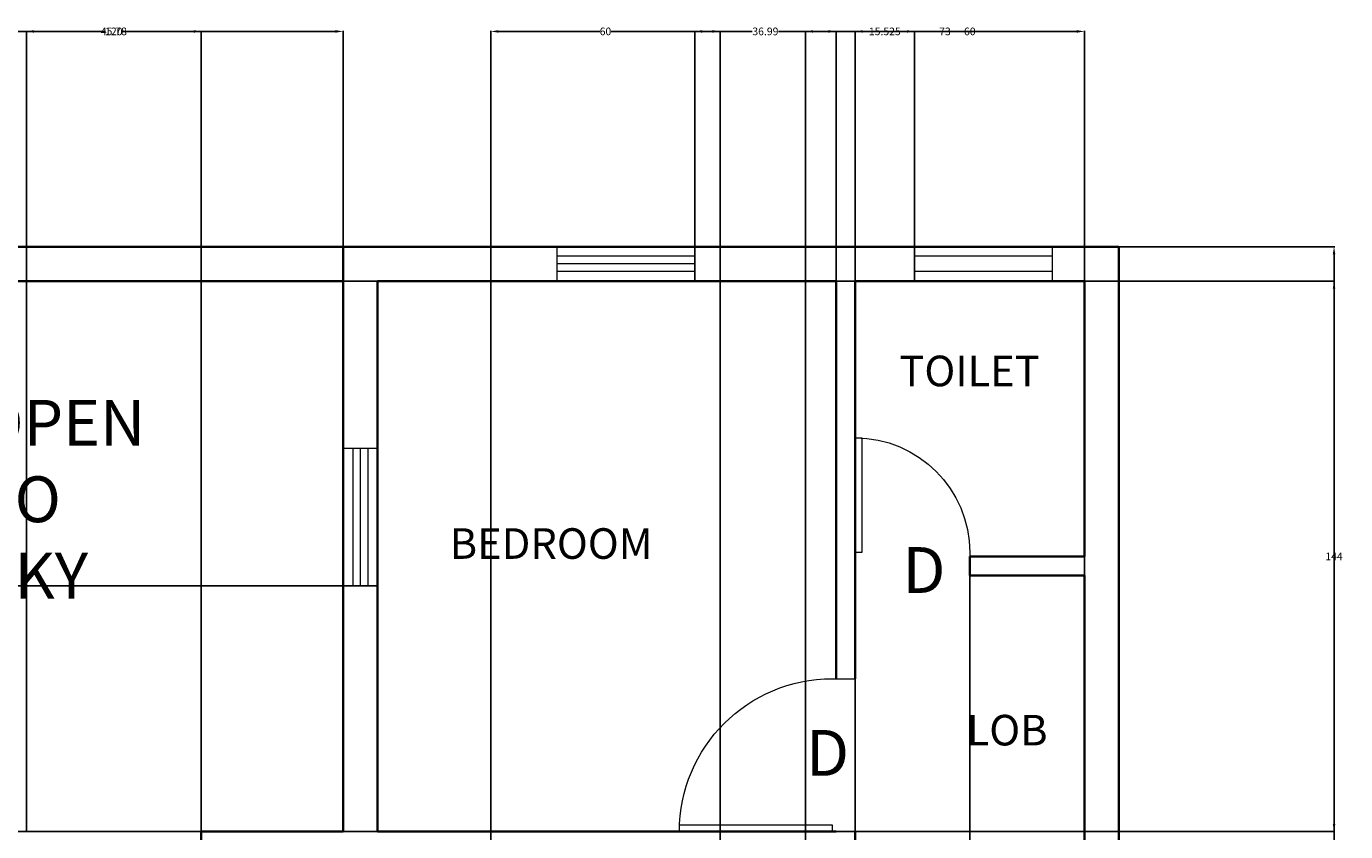
# Model space of a CAD drawing. Units: inches. Extents: x 190 to 836, y -241 to 999.
# Tile 9 of 9: x 491 to 836, y 789 to 999. Entities that reach past the tile are written whole.
import ezdxf

# ---------------------------------------------------------------- set-up
doc = ezdxf.new("R2010")
doc.units = ezdxf.units.IN
doc.header["$MEASUREMENT"] = 0
for name, color, linetype, lineweight in [('A-ANNO-DIMS', 2, 'Continuous', 18), ('A-ANNO-TEXT', 7, 'Continuous', 18), ('A-AREA-IDEN', 7, 'Continuous', 18), ('A-DOOR', 3, 'Continuous', 18), ('A-GLAZ', 4, 'Continuous', 18), ('A-WALL', 7, 'Continuous', 35)]:
    doc.layers.add(name, color=color, linetype=linetype, lineweight=lineweight)
doc.styles.get("Standard").update_dxf_attribs({"font": 'arial.ttf'})
doc.dimstyles.get("Standard").update_dxf_attribs({"dimtxt": 2, "dimasz": 2, "dimexe": 0.18, "dimexo": 0.0625, "dimgap": 0.09, "dimtad": 0, "dimtih": 1, "dimtoh": 1, "dimdec": 0, "dimzin": 0, "dimdsep": 46, "dimlunit": 3, "dimtxsty": 'Standard', "dimcen": 0.09, "dimadec": 0, "dimazin": 0, "dimtfac": 1, "dimtdec": 0, "dimtofl": 0, "dimtmove": 0, "dimatfit": 3, "dimfxl": 1, "dimtolj": 1, "dimtzin": 0, "dimarcsym": 0})

# ---------------------------------------------------------------- blocks, each defined once
blk = doc.blocks.new('*U2')
for p, q in [((0, 0), (0, 6)), ((40, 0), (40, 6))]:
    blk.add_line(p, q)
blk.add_lwpolyline([(0, 0), (0, -40), (1.75, -40), (1.75, 0)], close=True)
blk.add_arc((0, 0), 40, 270, 360)
blk = doc.blocks.new('*U3')
for p, q in [((-30, 0), (-30, -6)), ((0, 0), (0, -6))]:
    blk.add_line(p, q)
blk.add_lwpolyline([(0, 0), (0, 30), (-1.75, 30), (-1.75, 0)], close=True)
blk.add_arc((0, 0), 30, 90, 180)
blk = doc.blocks.new('WIN-36IN-9IN-3LINE')
for p, q in [((2.5, 36), (2.5, 0)), ((4.5, 36), (4.5, 0)), ((6.5, 36), (6.5, 0))]:
    blk.add_line(p, q)
blk.add_lwpolyline([(0, 0), (9, 0), (9, 36), (0, 36)], close=True)
blk = doc.blocks.new('WIN-36IN-9IN-2LINE')
for p, q in [((0, 6.5), (36, 6.5)), ((0, 2.5), (36, 2.5))]:
    blk.add_line(p, q)
blk.add_lwpolyline([(36, 0), (36, 9), (0, 9), (0, 0)], close=True)
blk = doc.blocks.new('*D18')
at = {"layer": 'A-ANNO-DIMS', "color": 0, "lineweight": -2, "transparency": 16777216}
for p, q in [((776.5, 941.53), (832.94, 941.53)), ((832.76, 939.53), (832.76, 403.14)), ((832.76, -135.47), (832.76, 400.92)), ((776.5, -137.47), (832.94, -137.47))]:
    blk.add_line(p, q, dxfattribs=at)
at = {"layer": 'A-ANNO-DIMS', "color": 0, "transparency": 16777216}
for points in [[(832.43, 939.53), (833.1, 939.53), (832.76, 941.53)], [(832.43, -135.47), (833.1, -135.47), (832.76, -137.47)]]:
    blk.add_solid(points, dxfattribs=at)
at = {"layer": 'Defpoints', "color": 0, "transparency": 16777216}
for p in [(776.44, 941.53), (832.76, 941.53), (776.44, -137.47)]:
    blk.add_point(p, dxfattribs=at)
at = {"layer": 'A-ANNO-DIMS', "color": 0, "transparency": 16777216, "insert": (832.76, 402.03), "char_height": 2, "attachment_point": 5}
blk.add_mtext('\\A1;1079', dxfattribs=at)
blk = doc.blocks.new('*D19')
at = {"layer": 'A-ANNO-DIMS', "color": 0, "lineweight": -2, "transparency": 16777216}
for p, q in [((453.44, 941.59), (453.44, 998.02)), ((455.44, 997.84), (511.24, 997.84)), ((571.44, 997.84), (515.64, 997.84)), ((573.44, 941.59), (573.44, 998.02))]:
    blk.add_line(p, q, dxfattribs=at)
at = {"layer": 'A-ANNO-DIMS', "color": 0, "transparency": 16777216}
for points in [[(455.44, 998.17), (455.44, 997.5), (453.44, 997.84)], [(571.44, 998.17), (571.44, 997.5), (573.44, 997.84)]]:
    blk.add_solid(points, dxfattribs=at)
at = {"layer": 'Defpoints', "color": 0, "transparency": 16777216}
for p in [(573.44, 997.84), (453.44, 941.53), (573.44, 941.53)]:
    blk.add_point(p, dxfattribs=at)
at = {"layer": 'A-ANNO-DIMS', "color": 0, "transparency": 16777216, "insert": (513.44, 997.84), "char_height": 2, "attachment_point": 5}
blk.add_mtext('\\A1;120', dxfattribs=at)
blk = doc.blocks.new('*D20')
at = {"layer": 'A-ANNO-DIMS', "color": 0, "lineweight": -2, "transparency": 16777216}
for p, q in [((490.55, 788.59), (490.55, 998.02)), ((492.55, 997.84), (509.94, 997.84)), ((534.33, 997.84), (516.95, 997.84)), ((536.33, 788.59), (536.33, 998.02))]:
    blk.add_line(p, q, dxfattribs=at)
at = {"layer": 'A-ANNO-DIMS', "color": 0, "transparency": 16777216}
for points in [[(492.55, 998.17), (492.55, 997.5), (490.55, 997.84)], [(534.33, 998.17), (534.33, 997.5), (536.33, 997.84)]]:
    blk.add_solid(points, dxfattribs=at)
at = {"layer": 'Defpoints', "color": 0, "transparency": 16777216}
for p in [(536.33, 997.84), (490.55, 788.53), (536.33, 788.53)]:
    blk.add_point(p, dxfattribs=at)
at = {"layer": 'A-ANNO-DIMS', "color": 0, "transparency": 16777216, "insert": (513.44, 997.84), "char_height": 2, "attachment_point": 5}
blk.add_mtext('\\A1;45.78', dxfattribs=at)
blk = doc.blocks.new('*D21')
at = {"layer": 'A-ANNO-DIMS', "color": 0, "lineweight": -2, "transparency": 16777216}
for p, q in [((776.5, 941.53), (832.94, 941.53)), ((832.76, 939.53), (832.76, 754.64)), ((832.76, 567.53), (832.76, 752.42)), ((767.5, 565.53), (832.94, 565.53))]:
    blk.add_line(p, q, dxfattribs=at)
at = {"layer": 'A-ANNO-DIMS', "color": 0, "transparency": 16777216}
for points in [[(832.43, 939.53), (833.1, 939.53), (832.76, 941.53)], [(832.43, 567.53), (833.1, 567.53), (832.76, 565.53)]]:
    blk.add_solid(points, dxfattribs=at)
at = {"layer": 'Defpoints', "color": 0, "transparency": 16777216}
for p in [(776.44, 941.53), (832.76, 941.53), (767.44, 565.53)]:
    blk.add_point(p, dxfattribs=at)
at = {"layer": 'A-ANNO-DIMS', "color": 0, "transparency": 16777216, "insert": (832.76, 753.53), "char_height": 2, "attachment_point": 5}
blk.add_mtext('\\A1;376', dxfattribs=at)
blk = doc.blocks.new('*D25')
at = {"layer": 'A-ANNO-DIMS', "color": 0, "lineweight": -2, "transparency": 16777216}
for p, q in [((444.5, 932.53), (832.94, 932.53)), ((832.76, 930.53), (832.76, 861.63)), ((832.76, 790.53), (832.76, 859.44)), ((444.5, 788.53), (832.94, 788.53))]:
    blk.add_line(p, q, dxfattribs=at)
at = {"layer": 'A-ANNO-DIMS', "color": 0, "transparency": 16777216}
for points in [[(832.43, 930.53), (833.1, 930.53), (832.76, 932.53)], [(832.43, 790.53), (833.1, 790.53), (832.76, 788.53)]]:
    blk.add_solid(points, dxfattribs=at)
at = {"layer": 'Defpoints', "color": 0, "transparency": 16777216}
for p in [(444.44, 932.53), (832.76, 932.53), (444.44, 788.53)]:
    blk.add_point(p, dxfattribs=at)
at = {"layer": 'A-ANNO-DIMS', "color": 0, "transparency": 16777216, "insert": (832.76, 860.53), "char_height": 2, "attachment_point": 5}
blk.add_mtext('\\A1;144', dxfattribs=at)
blk = doc.blocks.new('*D31')
at = {"layer": 'A-ANNO-DIMS', "color": 0, "lineweight": -2, "transparency": 16777216}
for p, q in [((707.44, 855.47), (707.44, -239.95)), ((737.44, 855.47), (737.44, -239.95)), ((709.44, -239.77), (720.92, -239.77)), ((735.44, -239.77), (723.96, -239.77))]:
    blk.add_line(p, q, dxfattribs=at)
at = {"layer": 'A-ANNO-DIMS', "color": 0, "transparency": 16777216}
for points in [[(709.44, -239.44), (709.44, -240.11), (707.44, -239.77)], [(735.44, -239.44), (735.44, -240.11), (737.44, -239.77)]]:
    blk.add_solid(points, dxfattribs=at)
at = {"layer": 'Defpoints', "color": 0, "transparency": 16777216}
for p in [(707.44, 855.53), (737.44, 855.53), (707.44, -239.77)]:
    blk.add_point(p, dxfattribs=at)
at = {"layer": 'A-ANNO-DIMS', "color": 0, "transparency": 16777216, "insert": (722.44, -239.77), "char_height": 2, "attachment_point": 5}
blk.add_mtext('\\A1;30', dxfattribs=at)
blk = doc.blocks.new('*D43')
at = {"layer": 'A-ANNO-DIMS', "color": 0, "lineweight": -2, "transparency": 16777216}
for p, q in [((694.44, -128.41), (694.44, 998.02)), ((696.44, 997.84), (729.43, 997.84)), ((765.44, 997.84), (732.45, 997.84)), ((767.44, -128.41), (767.44, 998.02))]:
    blk.add_line(p, q, dxfattribs=at)
at = {"layer": 'A-ANNO-DIMS', "color": 0, "transparency": 16777216}
for points in [[(696.44, 998.17), (696.44, 997.5), (694.44, 997.84)], [(765.44, 998.17), (765.44, 997.5), (767.44, 997.84)]]:
    blk.add_solid(points, dxfattribs=at)
at = {"layer": 'Defpoints', "color": 0, "transparency": 16777216}
for p in [(767.44, 997.84), (694.44, -128.47), (767.44, -128.47)]:
    blk.add_point(p, dxfattribs=at)
at = {"layer": 'A-ANNO-DIMS', "color": 0, "transparency": 16777216, "insert": (730.94, 997.84), "char_height": 2, "attachment_point": 5}
blk.add_mtext('\\A1;73', dxfattribs=at)
blk = doc.blocks.new('*D45')
at = {"layer": 'A-ANNO-DIMS', "color": 0, "lineweight": -2, "transparency": 16777216}
for p, q in [((612.1, 115.59), (612.1, 998.02)), ((614.1, 997.84), (640.58, 997.84)), ((670.1, 997.84), (643.62, 997.84)), ((672.1, 115.59), (672.1, 998.02))]:
    blk.add_line(p, q, dxfattribs=at)
at = {"layer": 'A-ANNO-DIMS', "color": 0, "transparency": 16777216}
for points in [[(614.1, 998.17), (614.1, 997.5), (612.1, 997.84)], [(670.1, 998.17), (670.1, 997.5), (672.1, 997.84)]]:
    blk.add_solid(points, dxfattribs=at)
at = {"layer": 'Defpoints', "color": 0, "transparency": 16777216}
for p in [(672.1, 997.84), (612.1, 115.53), (672.1, 115.53)]:
    blk.add_point(p, dxfattribs=at)
at = {"layer": 'A-ANNO-DIMS', "color": 0, "transparency": 16777216, "insert": (642.1, 997.84), "char_height": 2, "attachment_point": 5}
blk.add_mtext('\\A1;60', dxfattribs=at)
blk = doc.blocks.new('*D46')
at = {"layer": 'A-ANNO-DIMS', "color": 0, "lineweight": -2, "transparency": 16777216}
for p, q in [((707.44, 120.59), (707.44, 998.02)), ((709.44, 997.84), (735.92, 997.84)), ((765.44, 997.84), (738.97, 997.84)), ((767.44, 120.59), (767.44, 998.02))]:
    blk.add_line(p, q, dxfattribs=at)
at = {"layer": 'A-ANNO-DIMS', "color": 0, "transparency": 16777216}
for points in [[(709.44, 998.17), (709.44, 997.5), (707.44, 997.84)], [(765.44, 998.17), (765.44, 997.5), (767.44, 997.84)]]:
    blk.add_solid(points, dxfattribs=at)
at = {"layer": 'Defpoints', "color": 0, "transparency": 16777216}
for p in [(767.44, 997.84), (707.44, 120.53), (767.44, 120.53)]:
    blk.add_point(p, dxfattribs=at)
at = {"layer": 'A-ANNO-DIMS', "color": 0, "transparency": 16777216, "insert": (737.44, 997.84), "char_height": 2, "attachment_point": 5}
blk.add_mtext('\\A1;60', dxfattribs=at)
blk = doc.blocks.new('*D50')
at = {"layer": 'A-ANNO-DIMS', "color": 0, "lineweight": -2, "transparency": 16777216}
for p, q in [((665.45, 932.59), (665.45, 998.02)), ((667.45, 997.84), (680.48, 997.84)), ((700.44, 997.84), (687.41, 997.84)), ((702.44, 932.59), (702.44, 998.02))]:
    blk.add_line(p, q, dxfattribs=at)
at = {"layer": 'A-ANNO-DIMS', "color": 0, "transparency": 16777216}
for points in [[(667.45, 998.17), (667.45, 997.5), (665.45, 997.84)], [(700.44, 998.17), (700.44, 997.5), (702.44, 997.84)]]:
    blk.add_solid(points, dxfattribs=at)
at = {"layer": 'Defpoints', "color": 0, "transparency": 16777216}
for p in [(702.44, 997.84), (665.45, 932.53), (702.44, 932.53)]:
    blk.add_point(p, dxfattribs=at)
at = {"layer": 'A-ANNO-DIMS', "color": 0, "transparency": 16777216, "insert": (683.95, 997.84), "char_height": 2, "attachment_point": 5}
blk.add_mtext('\\A1;36.99', dxfattribs=at)
blk = doc.blocks.new('*D52')
at = {"layer": 'A-ANNO-DIMS', "color": 0, "lineweight": -2, "transparency": 16777216}
for p, q in [((582.38, 852.85), (193.96, 852.85)), ((194.14, 850.85), (194.14, 821.8)), ((194.14, 790.53), (194.14, 819.58)), ((582.38, 788.53), (193.96, 788.53))]:
    blk.add_line(p, q, dxfattribs=at)
at = {"layer": 'A-ANNO-DIMS', "color": 0, "transparency": 16777216}
for points in [[(193.8, 850.85), (194.47, 850.85), (194.14, 852.85)], [(193.8, 790.53), (194.47, 790.53), (194.14, 788.53)]]:
    blk.add_solid(points, dxfattribs=at)
at = {"layer": 'Defpoints', "color": 0, "transparency": 16777216}
for p in [(582.44, 852.85), (194.14, 788.53), (582.44, 788.53)]:
    blk.add_point(p, dxfattribs=at)
at = {"layer": 'A-ANNO-DIMS', "color": 0, "transparency": 16777216, "insert": (194.14, 820.69), "char_height": 2, "attachment_point": 5}
blk.add_mtext('\\A1;64.32', dxfattribs=at)
blk = doc.blocks.new('*D54')
at = {"layer": 'A-ANNO-DIMS', "color": 0, "lineweight": -2, "transparency": 16777216}
for p, q in [((707.44, 932.59), (707.44, 998.02)), ((709.44, 997.84), (711.05, 997.84)), ((720.97, 997.84), (719.36, 997.84)), ((722.97, 932.59), (722.97, 998.02))]:
    blk.add_line(p, q, dxfattribs=at)
at = {"layer": 'A-ANNO-DIMS', "color": 0, "transparency": 16777216}
for points in [[(709.44, 998.17), (709.44, 997.5), (707.44, 997.84)], [(720.97, 998.17), (720.97, 997.5), (722.97, 997.84)]]:
    blk.add_solid(points, dxfattribs=at)
at = {"layer": 'Defpoints', "color": 0, "transparency": 16777216}
for p in [(722.97, 997.84), (707.44, 932.53), (722.97, 932.53)]:
    blk.add_point(p, dxfattribs=at)
at = {"layer": 'A-ANNO-DIMS', "color": 0, "transparency": 16777216, "insert": (715.2, 997.84), "char_height": 2, "attachment_point": 5}
blk.add_mtext('\\A1;15.525', dxfattribs=at)

msp = doc.modelspace()

# ---------------------------------------------------------------- linework, layer by layer
at = {"layer": 'A-WALL'}
for p, q in [((453.4421, 941.5313), (573.4421, 941.5313)), ((573.4421, 941.5313), (776.4421, 941.5313)), ((573.4421, 788.5313), (573.4421, 941.5313)), ((776.4421, 941.5313), (776.4421, 556.5313)), ((453.4421, 932.5313), (573.4421, 932.5313)), ((582.4421, 932.5313), (702.4421, 932.5313)), ((582.4421, 788.5313), (582.4421, 932.5313)), ((702.4421, 828.5313), (702.4421, 932.5313)), ((707.4421, 932.5313), (767.4421, 932.5313)), ((707.4421, 828.5313), (707.4421, 932.5313)), ((767.4421, 932.5313), (767.4421, 860.5313)), ((767.4421, 860.5313), (737.4421, 860.5313)), ((737.4421, 860.5313), (737.4421, 855.5313)), ((767.4421, 855.5313), (737.4421, 855.5313)), ((767.4421, 855.5313), (767.4421, 565.5313)), ((573.4421, 788.5313), (536.3307, 788.5313)), ((536.3307, 788.5313), (536.3307, 732.9119)), ((702.4421, 788.5313), (582.4421, 788.5313)), ((707.4421, 779.5313), (707.4421, 788.5313))]:
    msp.add_line(p, q, dxfattribs=at)

# ---------------------------------------------------------------- block references
at = {"layer": 'A-DOOR', "xscale": -1}
for name, p, rotation in [('*U3', (707.4421, 861.5313), 360), ('*U2', (701.4421, 788.5313), 269.9999999999999)]:
    msp.add_blockref(name, p, dxfattribs=dict(at, rotation=rotation))
at = {"layer": 'A-GLAZ', "extrusion": (0, 0, -1), "zscale": -1, "rotation": 90.00000000000024}
msp.add_blockref('WIN-36IN-9IN-3LINE', (-629.4485, 932.5312), dxfattribs=at)
at = {"layer": 'A-GLAZ', "extrusion": (0, 0, -1), "zscale": -1}
for name, p in [('WIN-36IN-9IN-2LINE', (-758.9673, 932.531)), ('WIN-36IN-9IN-3LINE', (-582.4423, 852.851))]:
    msp.add_blockref(name, p, dxfattribs=at)

# ---------------------------------------------------------------- texts
at = {"layer": 'A-ANNO-TEXT', "char_height": 12, "attachment_point": 3}
for insert in [(731.0773, 862.9464), (705.8634, 815.1248)]:
    msp.add_mtext_dynamic_manual_height_columns('D', width=8.765037, gutter_width=1, heights=[0], dxfattribs=dict(at, insert=insert))
at = {"layer": 'A-AREA-IDEN'}
for s, width, insert, char_height, attachment_point in [('TOILET', 33.040256, (755.7407, 913.0231), 8, 3), ('OPEN TO SKY', 38.023659, (477.6605, 901.4652), 12, 1), ('BEDROOM', 33.040256, (654.438, 867.8794), 8, 3), ('LOB', 33.040256, (757.8021, 819.0683), 8, 3)]:
    msp.add_mtext_dynamic_manual_height_columns(s, width=width, gutter_width=1, heights=[0], dxfattribs=dict(at, insert=insert, char_height=char_height, attachment_point=attachment_point))

# ---------------------------------------------------------------- dimensions: what is measured, and where the dimension line sits
at = {"layer": 'A-ANNO-DIMS'}
for base, p1, p2, override, picture, middle in [((573.4421, 997.8363), (453.4421, 941.5313), (573.4421, 941.5313), {"dimdec": 0, "dimlfac": 1, "dimrnd": 0, "dimzin": 0, "dimdsep": 46, "dimlunit": 2}, '*D19', (513.4421, 997.8363)), ((536.3307, 997.8363), (490.5536, 788.5313), (536.3307, 788.5313), {"dimdec": 2, "dimlfac": 1, "dimrnd": 0, "dimzin": 0, "dimdsep": 46, "dimlunit": 2}, '*D20', (513.4421, 997.8363)), ((672.0998, 997.8363), (612.0998, 115.5313), (672.0998, 115.5313), {"dimdec": 0, "dimlfac": 1, "dimrnd": 0, "dimzin": 0, "dimdsep": 46, "dimlunit": 2}, '*D45', (642.0998, 997.8363)), ((702.4421, 997.8363), (665.4485, 932.5313), (702.4421, 932.5313), {"dimdec": 2, "dimlfac": 1, "dimrnd": 0, "dimzin": 0, "dimdsep": 46, "dimlunit": 2}, '*D50', (683.9453, 997.8363)), ((767.4421, 997.8363), (694.4376, -128.4687), (767.4421, -128.4687), {"dimdec": 0, "dimlfac": 1, "dimrnd": 0, "dimzin": 0, "dimdsep": 46, "dimlunit": 2}, '*D43', (730.9399, 997.8363)), ((767.4421, 997.8363), (707.4421, 120.5313), (767.4421, 120.5313), {"dimdec": 0, "dimlfac": 1, "dimrnd": 0, "dimzin": 0, "dimdsep": 46, "dimlunit": 2}, '*D46', (737.4421, 997.8363)), ((722.9668, 997.8363), (707.4421, 932.5313), (722.9668, 932.5313), {"dimdec": 3, "dimlfac": 1, "dimrnd": 0, "dimzin": 0, "dimdsep": 46, "dimlunit": 2}, '*D54', (715.2045, 997.8363)), ((707.4421, -239.7737), (737.4421, 855.5313), (707.4421, 855.5313), {"dimdec": 0, "dimlfac": 1, "dimrnd": 0, "dimzin": 0, "dimdsep": 46, "dimlunit": 2}, '*D31', (722.4421, -239.7737))]:
    dim = msp.add_linear_dim(base=base, p1=p1, p2=p2, dimstyle='Standard', override=override, dxfattribs=at)
    dim.commit()
    dim.dimension.update_dxf_attribs({"geometry": picture, "text_midpoint": middle})
for base, p1, p2, override, picture, middle in [((832.7634, 941.5313), (767.4421, 565.5313), (776.4421, 941.5313), {"dimdec": 0, "dimlfac": 1, "dimrnd": 0, "dimzin": 0, "dimdsep": 46, "dimlunit": 2}, '*D21', (832.7634, 753.5313)), ((832.7634, 941.5313), (776.4421, -137.4687), (776.4421, 941.5313), {"dimdec": 0, "dimlfac": 1, "dimrnd": 0, "dimzin": 0, "dimdsep": 46, "dimlunit": 2}, '*D18', (832.7634, 402.0313)), ((832.7634, 932.5313), (444.4421, 788.5313), (444.4421, 932.5313), {"dimdec": 0, "dimlfac": 1, "dimrnd": 0, "dimzin": 0, "dimdsep": 46, "dimlunit": 2}, '*D25', (832.7634, 860.5313)), ((194.1371, 788.5313), (582.4421, 852.851), (582.4421, 788.5313), {"dimdec": 2, "dimlfac": 1, "dimrnd": 0, "dimzin": 0, "dimdsep": 46, "dimlunit": 2}, '*D52', (194.1371, 820.6912))]:
    dim = msp.add_linear_dim(base=base, p1=p1, p2=p2, angle=90, dimstyle='Standard', override=override, dxfattribs=at)
    dim.commit()
    dim.dimension.update_dxf_attribs({"geometry": picture, "text_midpoint": middle})

doc.saveas('drawing.dxf')
